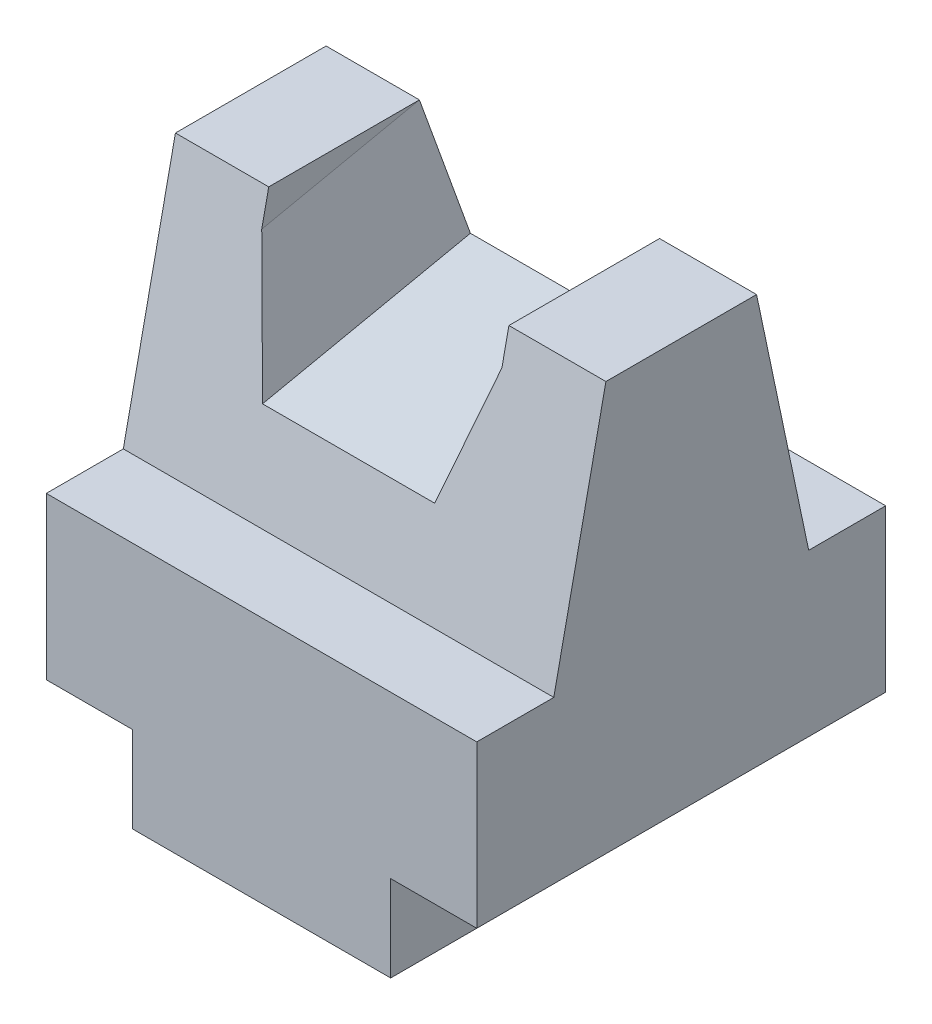
ISO-10303-21;
HEADER;
FILE_DESCRIPTION(('STEP AP214'),'2;1');
FILE_NAME('part.step','',(''),(''),'','','');
FILE_SCHEMA(('AUTOMOTIVE_DESIGN { 1 0 10303 214 1 1 1 1 }'));
ENDSEC;
DATA;
#1=APPLICATION_CONTEXT('core data for automotive mechanical design processes');
#2=APPLICATION_PROTOCOL_DEFINITION('international standard','automotive_design',2000,#1);
#3=PRODUCT_CONTEXT('',#1,'mechanical');
#4=PRODUCT('Part','Part','',(#3));
#5=PRODUCT_RELATED_PRODUCT_CATEGORY('part','',(#4));
#6=PRODUCT_DEFINITION_FORMATION('','',#4);
#7=PRODUCT_DEFINITION_CONTEXT('part definition',#1,'design');
#8=PRODUCT_DEFINITION('design','',#6,#7);
#9=PRODUCT_DEFINITION_SHAPE('','',#8);
#10=(LENGTH_UNIT() NAMED_UNIT(*) SI_UNIT(.MILLI.,.METRE.));
#11=(NAMED_UNIT(*) PLANE_ANGLE_UNIT() SI_UNIT($,.RADIAN.));
#12=(NAMED_UNIT(*) SI_UNIT($,.STERADIAN.) SOLID_ANGLE_UNIT());
#13=UNCERTAINTY_MEASURE_WITH_UNIT(LENGTH_MEASURE(1.E-05),#10,'distance_accuracy_value','');
#14=(GEOMETRIC_REPRESENTATION_CONTEXT(3) GLOBAL_UNCERTAINTY_ASSIGNED_CONTEXT((#13)) GLOBAL_UNIT_ASSIGNED_CONTEXT((#10,
#11,#12)) REPRESENTATION_CONTEXT('',''));
#15=CARTESIAN_POINT('',(0.,0.,0.));
#16=DIRECTION('',(0.,0.,1.));
#17=DIRECTION('',(1.,0.,0.));
#18=AXIS2_PLACEMENT_3D('',#15,#16,#17);
#19=CARTESIAN_POINT('',(-20.,23.,38.));
#20=DIRECTION('',(0.,-1.,0.));
#21=DIRECTION('',(0.,0.,-1.));
#22=AXIS2_PLACEMENT_3D('',#19,#20,#21);
#23=PLANE('',#22);
#24=DIRECTION('',(1.,0.,0.));
#25=VECTOR('',#24,1.);
#26=CARTESIAN_POINT('',(-20.,23.,12.));
#27=LINE('',#26,#25);
#28=CARTESIAN_POINT('',(10.9861695550396,23.,12.));
#29=VERTEX_POINT('',#28);
#30=CARTESIAN_POINT('',(20.,23.,12.));
#31=VERTEX_POINT('',#30);
#32=EDGE_CURVE('E200',#29,#31,#27,.T.);
#33=ORIENTED_EDGE('',*,*,#32,.F.);
#34=DIRECTION('',(0.,0.,1.));
#35=VECTOR('',#34,1.);
#36=CARTESIAN_POINT('',(10.9861695550396,23.,38.));
#37=LINE('',#36,#35);
#38=CARTESIAN_POINT('',(10.9861695550396,23.,26.));
#39=VERTEX_POINT('',#38);
#40=EDGE_CURVE('E167',#29,#39,#37,.T.);
#41=ORIENTED_EDGE('',*,*,#40,.T.);
#42=DIRECTION('',(-1.,0.,0.));
#43=VECTOR('',#42,1.);
#44=CARTESIAN_POINT('',(-20.,23.,26.));
#45=LINE('',#44,#43);
#46=CARTESIAN_POINT('',(20.,23.,26.));
#47=VERTEX_POINT('',#46);
#48=EDGE_CURVE('E178',#47,#39,#45,.T.);
#49=ORIENTED_EDGE('',*,*,#48,.F.);
#50=DIRECTION('',(0.,0.,-1.));
#51=VECTOR('',#50,1.);
#52=CARTESIAN_POINT('',(20.,23.,38.));
#53=LINE('',#52,#51);
#54=EDGE_CURVE('E199',#47,#31,#53,.T.);
#55=ORIENTED_EDGE('',*,*,#54,.T.);
#56=EDGE_LOOP('',(#33,#41,#49,#55));
#57=FACE_BOUND('',#56,.T.);
#58=ADVANCED_FACE('F43',(#57),#23,.F.);
#59=CARTESIAN_POINT('',(-46.,-1.44297082228117,6.85411140583554));
#60=DIRECTION('',(0.,0.206010481049842,-0.978549784986749));
#61=DIRECTION('',(0.,0.978549784986749,0.206010481049842));
#62=AXIS2_PLACEMENT_3D('',#59,#60,#61);
#63=PLANE('',#62);
#64=DIRECTION('',(-1.,0.,0.));
#65=VECTOR('',#64,1.);
#66=CARTESIAN_POINT('',(-46.,12.4045745886902,9.76938412393479));
#67=LINE('',#66,#65);
#68=CARTESIAN_POINT('',(7.18004102876759,12.4045745886902,9.76938412393478));
#69=VERTEX_POINT('',#68);
#70=CARTESIAN_POINT('',(-8.81995897123242,12.4045745886902,9.76938412393479));
#71=VERTEX_POINT('',#70);
#72=EDGE_CURVE('E279',#69,#71,#67,.T.);
#73=ORIENTED_EDGE('',*,*,#72,.F.);
#74=DIRECTION('',(0.331626211396949,0.923174496877331,0.194352525658385));
#75=VECTOR('',#74,1.);
#76=CARTESIAN_POINT('',(-3.09579074243356,-16.2010829237665,3.74714043710179));
#77=LINE('',#76,#75);
#78=EDGE_CURVE('E286',#69,#29,#77,.T.);
#79=ORIENTED_EDGE('',*,*,#78,.T.);
#80=ORIENTED_EDGE('',*,*,#32,.T.);
#81=DIRECTION('',(0.,-0.978549784986749,-0.206010481049842));
#82=VECTOR('',#81,1.);
#83=CARTESIAN_POINT('',(20.,28.2413793103448,13.1034482758621));
#84=LINE('',#83,#82);
#85=CARTESIAN_POINT('',(20.,0.,7.15789473684211));
#86=VERTEX_POINT('',#85);
#87=EDGE_CURVE('E271',#31,#86,#84,.T.);
#88=ORIENTED_EDGE('',*,*,#87,.T.);
#89=DIRECTION('',(1.,0.,0.));
#90=VECTOR('',#89,1.);
#91=CARTESIAN_POINT('',(-46.,0.,7.15789473684211));
#92=LINE('',#91,#90);
#93=CARTESIAN_POINT('',(-20.,0.,7.15789473684211));
#94=VERTEX_POINT('',#93);
#95=EDGE_CURVE('E273',#94,#86,#92,.T.);
#96=ORIENTED_EDGE('',*,*,#95,.F.);
#97=DIRECTION('',(0.,0.978549784986749,0.206010481049842));
#98=VECTOR('',#97,1.);
#99=CARTESIAN_POINT('',(-20.,28.2413793103448,13.1034482758621));
#100=LINE('',#99,#98);
#101=CARTESIAN_POINT('',(-20.,23.,12.));
#102=VERTEX_POINT('',#101);
#103=EDGE_CURVE('E267',#94,#102,#100,.T.);
#104=ORIENTED_EDGE('',*,*,#103,.T.);
#105=CARTESIAN_POINT('',(-11.3311099886057,23.,12.0000000000001));
#106=VERTEX_POINT('',#105);
#107=EDGE_CURVE('E198',#102,#106,#27,.T.);
#108=ORIENTED_EDGE('',*,*,#107,.T.);
#109=DIRECTION('',(-0.225923291600866,0.953249473358433,0.200684099654407));
#110=VECTOR('',#109,1.);
#111=CARTESIAN_POINT('',(-7.60327687289893,7.27096679968001,8.68862458940632));
#112=LINE('',#111,#110);
#113=EDGE_CURVE('E289',#71,#106,#112,.T.);
#114=ORIENTED_EDGE('',*,*,#113,.F.);
#115=EDGE_LOOP('',(#73,#79,#80,#88,#96,#104,#108,#114));
#116=FACE_BOUND('',#115,.T.);
#117=ADVANCED_FACE('F308',(#116),#63,.T.);
#118=CARTESIAN_POINT('',(-20.,23.,38.));
#119=DIRECTION('',(1.,0.,0.));
#120=DIRECTION('',(0.,1.,0.));
#121=AXIS2_PLACEMENT_3D('',#118,#119,#120);
#122=PLANE('',#121);
#123=DIRECTION('',(0.,-0.978549784986749,0.206010481049842));
#124=VECTOR('',#123,1.);
#125=CARTESIAN_POINT('',(-20.,20.5809018567639,26.5092838196287));
#126=LINE('',#125,#124);
#127=CARTESIAN_POINT('',(-20.,23.,26.));
#128=VERTEX_POINT('',#127);
#129=CARTESIAN_POINT('',(-20.,0.,30.8421052631579));
#130=VERTEX_POINT('',#129);
#131=EDGE_CURVE('E264',#128,#130,#126,.T.);
#132=ORIENTED_EDGE('',*,*,#131,.F.);
#133=DIRECTION('',(0.,0.,-1.));
#134=VECTOR('',#133,1.);
#135=CARTESIAN_POINT('',(-20.,23.,38.));
#136=LINE('',#135,#134);
#137=EDGE_CURVE('E201',#128,#102,#136,.T.);
#138=ORIENTED_EDGE('',*,*,#137,.T.);
#139=ORIENTED_EDGE('',*,*,#103,.F.);
#140=DIRECTION('',(0.,0.,-1.));
#141=VECTOR('',#140,1.);
#142=CARTESIAN_POINT('',(-20.,0.,38.));
#143=LINE('',#142,#141);
#144=CARTESIAN_POINT('',(-20.,0.,0.));
#145=VERTEX_POINT('',#144);
#146=EDGE_CURVE('E265',#94,#145,#143,.T.);
#147=ORIENTED_EDGE('',*,*,#146,.T.);
#148=DIRECTION('',(0.,-1.,0.));
#149=VECTOR('',#148,1.);
#150=CARTESIAN_POINT('',(-20.,23.,0.));
#151=LINE('',#150,#149);
#152=CARTESIAN_POINT('',(-20.,-15.,0.));
#153=VERTEX_POINT('',#152);
#154=EDGE_CURVE('E211',#145,#153,#151,.T.);
#155=ORIENTED_EDGE('',*,*,#154,.T.);
#156=DIRECTION('',(0.,0.,1.));
#157=VECTOR('',#156,1.);
#158=CARTESIAN_POINT('',(-20.,-15.,0.));
#159=LINE('',#158,#157);
#160=CARTESIAN_POINT('',(-20.,-15.,38.));
#161=VERTEX_POINT('',#160);
#162=EDGE_CURVE('E224',#153,#161,#159,.T.);
#163=ORIENTED_EDGE('',*,*,#162,.T.);
#164=DIRECTION('',(0.,-1.,0.));
#165=VECTOR('',#164,1.);
#166=CARTESIAN_POINT('',(-20.,23.,38.));
#167=LINE('',#166,#165);
#168=CARTESIAN_POINT('',(-20.,0.,38.));
#169=VERTEX_POINT('',#168);
#170=EDGE_CURVE('E218',#169,#161,#167,.T.);
#171=ORIENTED_EDGE('',*,*,#170,.F.);
#172=DIRECTION('',(0.,0.,-1.));
#173=VECTOR('',#172,1.);
#174=CARTESIAN_POINT('',(-20.,0.,38.));
#175=LINE('',#174,#173);
#176=EDGE_CURVE('E254',#169,#130,#175,.T.);
#177=ORIENTED_EDGE('',*,*,#176,.T.);
#178=EDGE_LOOP('',(#132,#138,#139,#147,#155,#163,#171,#177));
#179=FACE_BOUND('',#178,.T.);
#180=ADVANCED_FACE('F313',(#179),#122,.F.);
#181=CARTESIAN_POINT('',(20.,23.,38.));
#182=DIRECTION('',(-1.,0.,0.));
#183=DIRECTION('',(0.,-1.,0.));
#184=AXIS2_PLACEMENT_3D('',#181,#182,#183);
#185=PLANE('',#184);
#186=DIRECTION('',(0.,0.978549784986749,-0.206010481049842));
#187=VECTOR('',#186,1.);
#188=CARTESIAN_POINT('',(20.,20.5809018567639,26.5092838196287));
#189=LINE('',#188,#187);
#190=CARTESIAN_POINT('',(20.,0.,30.8421052631579));
#191=VERTEX_POINT('',#190);
#192=EDGE_CURVE('E270',#191,#47,#189,.T.);
#193=ORIENTED_EDGE('',*,*,#192,.F.);
#194=DIRECTION('',(0.,0.,1.));
#195=VECTOR('',#194,1.);
#196=CARTESIAN_POINT('',(20.,0.,38.));
#197=LINE('',#196,#195);
#198=CARTESIAN_POINT('',(20.,0.,38.));
#199=VERTEX_POINT('',#198);
#200=EDGE_CURVE('E188',#191,#199,#197,.T.);
#201=ORIENTED_EDGE('',*,*,#200,.T.);
#202=DIRECTION('',(0.,1.,0.));
#203=VECTOR('',#202,1.);
#204=CARTESIAN_POINT('',(20.,23.,38.));
#205=LINE('',#204,#203);
#206=CARTESIAN_POINT('',(20.,-15.,38.));
#207=VERTEX_POINT('',#206);
#208=EDGE_CURVE('E209',#207,#199,#205,.T.);
#209=ORIENTED_EDGE('',*,*,#208,.F.);
#210=DIRECTION('',(0.,0.,1.));
#211=VECTOR('',#210,1.);
#212=CARTESIAN_POINT('',(20.,-15.,0.));
#213=LINE('',#212,#211);
#214=CARTESIAN_POINT('',(20.,-15.,0.));
#215=VERTEX_POINT('',#214);
#216=EDGE_CURVE('E245',#215,#207,#213,.T.);
#217=ORIENTED_EDGE('',*,*,#216,.F.);
#218=DIRECTION('',(0.,1.,0.));
#219=VECTOR('',#218,1.);
#220=CARTESIAN_POINT('',(20.,23.,0.));
#221=LINE('',#220,#219);
#222=CARTESIAN_POINT('',(20.,0.,0.));
#223=VERTEX_POINT('',#222);
#224=EDGE_CURVE('E213',#215,#223,#221,.T.);
#225=ORIENTED_EDGE('',*,*,#224,.T.);
#226=DIRECTION('',(0.,0.,1.));
#227=VECTOR('',#226,1.);
#228=CARTESIAN_POINT('',(20.,0.,38.));
#229=LINE('',#228,#227);
#230=EDGE_CURVE('E191',#223,#86,#229,.T.);
#231=ORIENTED_EDGE('',*,*,#230,.T.);
#232=ORIENTED_EDGE('',*,*,#87,.F.);
#233=ORIENTED_EDGE('',*,*,#54,.F.);
#234=EDGE_LOOP('',(#193,#201,#209,#217,#225,#231,#232,#233));
#235=FACE_BOUND('',#234,.T.);
#236=ADVANCED_FACE('F44',(#235),#185,.F.);
#237=CARTESIAN_POINT('',(-11.3311099886057,23.,26.));
#238=VERTEX_POINT('',#237);
#239=EDGE_CURVE('E195',#238,#128,#45,.T.);
#240=ORIENTED_EDGE('',*,*,#239,.F.);
#241=DIRECTION('',(0.,0.,-1.));
#242=VECTOR('',#241,1.);
#243=CARTESIAN_POINT('',(-11.3311099886057,23.,38.));
#244=LINE('',#243,#242);
#245=EDGE_CURVE('E180',#238,#106,#244,.T.);
#246=ORIENTED_EDGE('',*,*,#245,.T.);
#247=ORIENTED_EDGE('',*,*,#107,.F.);
#248=ORIENTED_EDGE('',*,*,#137,.F.);
#249=EDGE_LOOP('',(#240,#246,#247,#248));
#250=FACE_BOUND('',#249,.T.);
#251=ADVANCED_FACE('F297',(#250),#23,.F.);
#252=CARTESIAN_POINT('',(0.,0.,38.));
#253=DIRECTION('',(0.,0.,1.));
#254=DIRECTION('',(1.,0.,0.));
#255=AXIS2_PLACEMENT_3D('',#252,#253,#254);
#256=PLANE('',#255);
#257=DIRECTION('',(1.,0.,0.));
#258=VECTOR('',#257,1.);
#259=CARTESIAN_POINT('',(-46.,0.,38.));
#260=LINE('',#259,#258);
#261=EDGE_CURVE('E283',#169,#199,#260,.T.);
#262=ORIENTED_EDGE('',*,*,#261,.F.);
#263=ORIENTED_EDGE('',*,*,#170,.T.);
#264=DIRECTION('',(1.,0.,0.));
#265=VECTOR('',#264,1.);
#266=CARTESIAN_POINT('',(0.,-15.,38.));
#267=LINE('',#266,#265);
#268=CARTESIAN_POINT('',(-12.,-15.,38.));
#269=VERTEX_POINT('',#268);
#270=EDGE_CURVE('E233',#161,#269,#267,.T.);
#271=ORIENTED_EDGE('',*,*,#270,.T.);
#272=DIRECTION('',(0.,1.,0.));
#273=VECTOR('',#272,1.);
#274=CARTESIAN_POINT('',(-12.,0.,38.));
#275=LINE('',#274,#273);
#276=CARTESIAN_POINT('',(-12.,-23.,38.));
#277=VERTEX_POINT('',#276);
#278=EDGE_CURVE('E229',#277,#269,#275,.T.);
#279=ORIENTED_EDGE('',*,*,#278,.F.);
#280=DIRECTION('',(1.,0.,0.));
#281=VECTOR('',#280,1.);
#282=CARTESIAN_POINT('',(-20.,-23.,38.));
#283=LINE('',#282,#281);
#284=CARTESIAN_POINT('',(12.,-23.,38.));
#285=VERTEX_POINT('',#284);
#286=EDGE_CURVE('E206',#277,#285,#283,.T.);
#287=ORIENTED_EDGE('',*,*,#286,.T.);
#288=DIRECTION('',(0.,-1.,0.));
#289=VECTOR('',#288,1.);
#290=CARTESIAN_POINT('',(12.,-23.,38.));
#291=LINE('',#290,#289);
#292=CARTESIAN_POINT('',(12.,-15.,38.));
#293=VERTEX_POINT('',#292);
#294=EDGE_CURVE('E248',#293,#285,#291,.T.);
#295=ORIENTED_EDGE('',*,*,#294,.F.);
#296=DIRECTION('',(-1.,0.,0.));
#297=VECTOR('',#296,1.);
#298=CARTESIAN_POINT('',(12.,-15.,38.));
#299=LINE('',#298,#297);
#300=EDGE_CURVE('E252',#207,#293,#299,.T.);
#301=ORIENTED_EDGE('',*,*,#300,.F.);
#302=ORIENTED_EDGE('',*,*,#208,.T.);
#303=EDGE_LOOP('',(#262,#263,#271,#279,#287,#295,#301,#302));
#304=FACE_BOUND('',#303,.T.);
#305=ADVANCED_FACE('F324',(#304),#256,.T.);
#306=CARTESIAN_POINT('',(0.,0.,0.));
#307=DIRECTION('',(0.,0.,1.));
#308=DIRECTION('',(1.,0.,0.));
#309=AXIS2_PLACEMENT_3D('',#306,#307,#308);
#310=PLANE('',#309);
#311=ORIENTED_EDGE('',*,*,#154,.F.);
#312=DIRECTION('',(1.,0.,0.));
#313=VECTOR('',#312,1.);
#314=CARTESIAN_POINT('',(-46.,0.,0.));
#315=LINE('',#314,#313);
#316=EDGE_CURVE('E280',#145,#223,#315,.T.);
#317=ORIENTED_EDGE('',*,*,#316,.T.);
#318=ORIENTED_EDGE('',*,*,#224,.F.);
#319=DIRECTION('',(-1.,0.,0.));
#320=VECTOR('',#319,1.);
#321=CARTESIAN_POINT('',(12.,-15.,0.));
#322=LINE('',#321,#320);
#323=CARTESIAN_POINT('',(12.,-15.,0.));
#324=VERTEX_POINT('',#323);
#325=EDGE_CURVE('E253',#215,#324,#322,.T.);
#326=ORIENTED_EDGE('',*,*,#325,.T.);
#327=DIRECTION('',(0.,-1.,0.));
#328=VECTOR('',#327,1.);
#329=CARTESIAN_POINT('',(12.,-23.,0.));
#330=LINE('',#329,#328);
#331=CARTESIAN_POINT('',(12.,-23.,0.));
#332=VERTEX_POINT('',#331);
#333=EDGE_CURVE('E244',#324,#332,#330,.T.);
#334=ORIENTED_EDGE('',*,*,#333,.T.);
#335=DIRECTION('',(1.,0.,0.));
#336=VECTOR('',#335,1.);
#337=CARTESIAN_POINT('',(-20.,-23.,0.));
#338=LINE('',#337,#336);
#339=CARTESIAN_POINT('',(-12.,-23.,0.));
#340=VERTEX_POINT('',#339);
#341=EDGE_CURVE('E210',#340,#332,#338,.T.);
#342=ORIENTED_EDGE('',*,*,#341,.F.);
#343=DIRECTION('',(0.,1.,0.));
#344=VECTOR('',#343,1.);
#345=CARTESIAN_POINT('',(-12.,0.,0.));
#346=LINE('',#345,#344);
#347=CARTESIAN_POINT('',(-12.,-15.,0.));
#348=VERTEX_POINT('',#347);
#349=EDGE_CURVE('E230',#340,#348,#346,.T.);
#350=ORIENTED_EDGE('',*,*,#349,.T.);
#351=DIRECTION('',(1.,0.,0.));
#352=VECTOR('',#351,1.);
#353=CARTESIAN_POINT('',(0.,-15.,0.));
#354=LINE('',#353,#352);
#355=EDGE_CURVE('E234',#153,#348,#354,.T.);
#356=ORIENTED_EDGE('',*,*,#355,.F.);
#357=EDGE_LOOP('',(#311,#317,#318,#326,#334,#342,#350,#356));
#358=FACE_BOUND('',#357,.T.);
#359=ADVANCED_FACE('F335',(#358),#310,.F.);
#360=CARTESIAN_POINT('',(-20.,-23.,38.));
#361=DIRECTION('',(0.,1.,0.));
#362=DIRECTION('',(0.,0.,1.));
#363=AXIS2_PLACEMENT_3D('',#360,#361,#362);
#364=PLANE('',#363);
#365=ORIENTED_EDGE('',*,*,#341,.T.);
#366=DIRECTION('',(0.,0.,1.));
#367=VECTOR('',#366,1.);
#368=CARTESIAN_POINT('',(12.,-23.,0.));
#369=LINE('',#368,#367);
#370=EDGE_CURVE('E240',#332,#285,#369,.T.);
#371=ORIENTED_EDGE('',*,*,#370,.T.);
#372=ORIENTED_EDGE('',*,*,#286,.F.);
#373=DIRECTION('',(0.,0.,1.));
#374=VECTOR('',#373,1.);
#375=CARTESIAN_POINT('',(-12.,-23.,0.));
#376=LINE('',#375,#374);
#377=EDGE_CURVE('E228',#340,#277,#376,.T.);
#378=ORIENTED_EDGE('',*,*,#377,.F.);
#379=EDGE_LOOP('',(#365,#371,#372,#378));
#380=FACE_BOUND('',#379,.T.);
#381=ADVANCED_FACE('F367',(#380),#364,.F.);
#382=CARTESIAN_POINT('',(0.,-15.,0.));
#383=DIRECTION('',(0.,-1.,0.));
#384=DIRECTION('',(0.,0.,-1.));
#385=AXIS2_PLACEMENT_3D('',#382,#383,#384);
#386=PLANE('',#385);
#387=ORIENTED_EDGE('',*,*,#270,.F.);
#388=ORIENTED_EDGE('',*,*,#162,.F.);
#389=ORIENTED_EDGE('',*,*,#355,.T.);
#390=DIRECTION('',(0.,0.,1.));
#391=VECTOR('',#390,1.);
#392=CARTESIAN_POINT('',(-12.,-15.,0.));
#393=LINE('',#392,#391);
#394=EDGE_CURVE('E216',#348,#269,#393,.T.);
#395=ORIENTED_EDGE('',*,*,#394,.T.);
#396=EDGE_LOOP('',(#387,#388,#389,#395));
#397=FACE_BOUND('',#396,.T.);
#398=ADVANCED_FACE('F373',(#397),#386,.T.);
#399=CARTESIAN_POINT('',(-12.,0.,0.));
#400=DIRECTION('',(1.,0.,0.));
#401=DIRECTION('',(0.,0.,-1.));
#402=AXIS2_PLACEMENT_3D('',#399,#400,#401);
#403=PLANE('',#402);
#404=ORIENTED_EDGE('',*,*,#278,.T.);
#405=ORIENTED_EDGE('',*,*,#394,.F.);
#406=ORIENTED_EDGE('',*,*,#349,.F.);
#407=ORIENTED_EDGE('',*,*,#377,.T.);
#408=EDGE_LOOP('',(#404,#405,#406,#407));
#409=FACE_BOUND('',#408,.T.);
#410=ADVANCED_FACE('F377',(#409),#403,.F.);
#411=CARTESIAN_POINT('',(12.,-23.,0.));
#412=DIRECTION('',(-1.,0.,0.));
#413=DIRECTION('',(0.,0.,1.));
#414=AXIS2_PLACEMENT_3D('',#411,#412,#413);
#415=PLANE('',#414);
#416=ORIENTED_EDGE('',*,*,#294,.T.);
#417=ORIENTED_EDGE('',*,*,#370,.F.);
#418=ORIENTED_EDGE('',*,*,#333,.F.);
#419=DIRECTION('',(0.,0.,1.));
#420=VECTOR('',#419,1.);
#421=CARTESIAN_POINT('',(12.,-15.,0.));
#422=LINE('',#421,#420);
#423=EDGE_CURVE('E242',#324,#293,#422,.T.);
#424=ORIENTED_EDGE('',*,*,#423,.T.);
#425=EDGE_LOOP('',(#416,#417,#418,#424));
#426=FACE_BOUND('',#425,.T.);
#427=ADVANCED_FACE('F382',(#426),#415,.F.);
#428=CARTESIAN_POINT('',(12.,-15.,0.));
#429=DIRECTION('',(0.,1.,0.));
#430=DIRECTION('',(0.,0.,1.));
#431=AXIS2_PLACEMENT_3D('',#428,#429,#430);
#432=PLANE('',#431);
#433=ORIENTED_EDGE('',*,*,#300,.T.);
#434=ORIENTED_EDGE('',*,*,#423,.F.);
#435=ORIENTED_EDGE('',*,*,#325,.F.);
#436=ORIENTED_EDGE('',*,*,#216,.T.);
#437=EDGE_LOOP('',(#433,#434,#435,#436));
#438=FACE_BOUND('',#437,.T.);
#439=ADVANCED_FACE('F327',(#438),#432,.F.);
#440=CARTESIAN_POINT('',(-46.,0.,0.));
#441=DIRECTION('',(0.,-1.,0.));
#442=DIRECTION('',(0.,0.,-1.));
#443=AXIS2_PLACEMENT_3D('',#440,#441,#442);
#444=PLANE('',#443);
#445=ORIENTED_EDGE('',*,*,#95,.T.);
#446=ORIENTED_EDGE('',*,*,#230,.F.);
#447=ORIENTED_EDGE('',*,*,#316,.F.);
#448=ORIENTED_EDGE('',*,*,#146,.F.);
#449=EDGE_LOOP('',(#445,#446,#447,#448));
#450=FACE_BOUND('',#449,.T.);
#451=ADVANCED_FACE('F333',(#450),#444,.F.);
#452=CARTESIAN_POINT('',(-46.,0.,0.));
#453=DIRECTION('',(0.,-1.,0.));
#454=DIRECTION('',(0.,0.,-1.));
#455=AXIS2_PLACEMENT_3D('',#452,#453,#454);
#456=PLANE('',#455);
#457=ORIENTED_EDGE('',*,*,#261,.T.);
#458=ORIENTED_EDGE('',*,*,#200,.F.);
#459=DIRECTION('',(1.,0.,0.));
#460=VECTOR('',#459,1.);
#461=CARTESIAN_POINT('',(-46.,0.,30.8421052631579));
#462=LINE('',#461,#460);
#463=EDGE_CURVE('E272',#130,#191,#462,.T.);
#464=ORIENTED_EDGE('',*,*,#463,.F.);
#465=ORIENTED_EDGE('',*,*,#176,.F.);
#466=EDGE_LOOP('',(#457,#458,#464,#465));
#467=FACE_BOUND('',#466,.T.);
#468=ADVANCED_FACE('F320',(#467),#456,.F.);
#469=CARTESIAN_POINT('',(-46.,6.21750663129974,29.5331564986737));
#470=DIRECTION('',(0.,0.206010481049842,0.978549784986749));
#471=DIRECTION('',(0.,-0.978549784986749,0.206010481049842));
#472=AXIS2_PLACEMENT_3D('',#469,#470,#471);
#473=PLANE('',#472);
#474=DIRECTION('',(0.,0.978549784986749,-0.206010481049842));
#475=VECTOR('',#474,1.);
#476=CARTESIAN_POINT('',(10.9861695550396,6.21750663129974,29.5331564986737));
#477=LINE('',#476,#475);
#478=CARTESIAN_POINT('',(10.9861695550396,19.9159420289855,26.6492753623189));
#479=VERTEX_POINT('',#478);
#480=EDGE_CURVE('E163',#479,#39,#477,.T.);
#481=ORIENTED_EDGE('',*,*,#480,.F.);
#482=DIRECTION('',(-0.306227170808341,-0.931538751639651,0.196113421397821));
#483=VECTOR('',#482,1.);
#484=CARTESIAN_POINT('',(1.56144510730515,-8.75393734003065,32.6850394400065));
#485=LINE('',#484,#483);
#486=CARTESIAN_POINT('',(7.18004102876758,8.33775252155425,29.0867889428307));
#487=VERTEX_POINT('',#486);
#488=EDGE_CURVE('E51',#479,#487,#485,.T.);
#489=ORIENTED_EDGE('',*,*,#488,.T.);
#490=DIRECTION('',(1.,0.,0.));
#491=VECTOR('',#490,1.);
#492=CARTESIAN_POINT('',(-46.,8.33775252155425,29.0867889428307));
#493=LINE('',#492,#491);
#494=CARTESIAN_POINT('',(-8.81995897123242,8.33775252155425,29.0867889428307));
#495=VERTEX_POINT('',#494);
#496=EDGE_CURVE('E11',#495,#487,#493,.T.);
#497=ORIENTED_EDGE('',*,*,#496,.F.);
#498=DIRECTION('',(0.207609852951133,-0.957228858180155,0.201521864880033));
#499=VECTOR('',#498,1.);
#500=CARTESIAN_POINT('',(-9.98245570132067,13.6976880051677,27.9583814725963));
#501=LINE('',#500,#499);
#502=CARTESIAN_POINT('',(-11.3311099886057,19.9159420289855,26.6492753623188));
#503=VERTEX_POINT('',#502);
#504=EDGE_CURVE('E183',#503,#495,#501,.T.);
#505=ORIENTED_EDGE('',*,*,#504,.F.);
#506=DIRECTION('',(0.,-0.978549784986749,0.206010481049842));
#507=VECTOR('',#506,1.);
#508=CARTESIAN_POINT('',(-11.3311099886057,6.21750663129974,29.5331564986737));
#509=LINE('',#508,#507);
#510=EDGE_CURVE('E66',#238,#503,#509,.T.);
#511=ORIENTED_EDGE('',*,*,#510,.F.);
#512=ORIENTED_EDGE('',*,*,#239,.T.);
#513=ORIENTED_EDGE('',*,*,#131,.T.);
#514=ORIENTED_EDGE('',*,*,#463,.T.);
#515=ORIENTED_EDGE('',*,*,#192,.T.);
#516=ORIENTED_EDGE('',*,*,#48,.T.);
#517=EDGE_LOOP('',(#481,#489,#497,#505,#511,#512,#513,#514,#515,#516));
#518=FACE_BOUND('',#517,.T.);
#519=ADVANCED_FACE('F176',(#518),#473,.T.);
#520=CARTESIAN_POINT('',(0.,2.9280924603975,54.7826742333253));
#521=DIRECTION('',(0.,-0.978549784986749,-0.206010481049842));
#522=DIRECTION('',(0.,0.206010481049842,-0.978549784986749));
#523=AXIS2_PLACEMENT_3D('',#520,#521,#522);
#524=PLANE('',#523);
#525=ORIENTED_EDGE('',*,*,#72,.T.);
#526=DIRECTION('',(0.,0.206010481049842,-0.978549784986749));
#527=VECTOR('',#526,1.);
#528=CARTESIAN_POINT('',(-8.81995897123242,2.9280924603975,54.7826742333253));
#529=LINE('',#528,#527);
#530=EDGE_CURVE('E59',#495,#71,#529,.T.);
#531=ORIENTED_EDGE('',*,*,#530,.F.);
#532=ORIENTED_EDGE('',*,*,#496,.T.);
#533=DIRECTION('',(0.,0.206010481049842,-0.978549784986749));
#534=VECTOR('',#533,1.);
#535=CARTESIAN_POINT('',(7.18004102876758,2.9280924603975,54.7826742333253));
#536=LINE('',#535,#534);
#537=EDGE_CURVE('E168',#487,#69,#536,.T.);
#538=ORIENTED_EDGE('',*,*,#537,.T.);
#539=EDGE_LOOP('',(#525,#531,#532,#538));
#540=FACE_BOUND('',#539,.T.);
#541=ADVANCED_FACE('F339',(#540),#524,.F.);
#542=CARTESIAN_POINT('',(1.96310268549916,-11.5947174526044,51.7252405674301));
#543=DIRECTION('',(-0.943410862728698,0.324512757858455,0.0683184753386221));
#544=DIRECTION('',(-0.325272736954854,-0.945620244386666,0.));
#545=AXIS2_PLACEMENT_3D('',#542,#543,#544);
#546=PLANE('',#545);
#547=ORIENTED_EDGE('',*,*,#537,.F.);
#548=ORIENTED_EDGE('',*,*,#488,.F.);
#549=DIRECTION('',(0.,0.206010481049842,-0.978549784986749));
#550=VECTOR('',#549,1.);
#551=CARTESIAN_POINT('',(10.9861695550396,13.5235178717073,57.0132901093905));
#552=LINE('',#551,#550);
#553=EDGE_CURVE('E161',#479,#29,#552,.T.);
#554=ORIENTED_EDGE('',*,*,#553,.T.);
#555=ORIENTED_EDGE('',*,*,#78,.F.);
#556=EDGE_LOOP('',(#547,#548,#554,#555));
#557=FACE_BOUND('',#556,.T.);
#558=ADVANCED_FACE('F181',(#557),#546,.T.);
#559=CARTESIAN_POINT('',(-5.25537552326151,-12.1121332305575,51.6163109299663));
#560=DIRECTION('',(-0.974145095102485,-0.221077188419526,-0.0465425659830581));
#561=DIRECTION('',(0.22131702800492,-0.975201914023485,0.));
#562=AXIS2_PLACEMENT_3D('',#559,#560,#561);
#563=PLANE('',#562);
#564=ORIENTED_EDGE('',*,*,#113,.T.);
#565=DIRECTION('',(0.,0.206010481049842,-0.978549784986749));
#566=VECTOR('',#565,1.);
#567=CARTESIAN_POINT('',(-11.3311099886057,13.5235178717073,57.0132901093905));
#568=LINE('',#567,#566);
#569=EDGE_CURVE('E173',#503,#106,#568,.T.);
#570=ORIENTED_EDGE('',*,*,#569,.F.);
#571=ORIENTED_EDGE('',*,*,#504,.T.);
#572=ORIENTED_EDGE('',*,*,#530,.T.);
#573=EDGE_LOOP('',(#564,#570,#571,#572));
#574=FACE_BOUND('',#573,.T.);
#575=ADVANCED_FACE('F302',(#574),#563,.F.);
#576=CARTESIAN_POINT('',(-11.3311099886057,13.5235178717073,57.0132901093905));
#577=DIRECTION('',(-1.,0.,0.));
#578=DIRECTION('',(0.,0.,1.));
#579=AXIS2_PLACEMENT_3D('',#576,#577,#578);
#580=PLANE('',#579);
#581=ORIENTED_EDGE('',*,*,#510,.T.);
#582=ORIENTED_EDGE('',*,*,#569,.T.);
#583=ORIENTED_EDGE('',*,*,#245,.F.);
#584=EDGE_LOOP('',(#581,#582,#583));
#585=FACE_BOUND('',#584,.T.);
#586=ADVANCED_FACE('F492',(#585),#580,.F.);
#587=CARTESIAN_POINT('',(10.9861695550396,13.5235178717073,57.0132901093905));
#588=DIRECTION('',(1.,0.,0.));
#589=DIRECTION('',(0.,0.,-1.));
#590=AXIS2_PLACEMENT_3D('',#587,#588,#589);
#591=PLANE('',#590);
#592=ORIENTED_EDGE('',*,*,#553,.F.);
#593=ORIENTED_EDGE('',*,*,#480,.T.);
#594=ORIENTED_EDGE('',*,*,#40,.F.);
#595=EDGE_LOOP('',(#592,#593,#594));
#596=FACE_BOUND('',#595,.T.);
#597=ADVANCED_FACE('F162',(#596),#591,.F.);
#598=CLOSED_SHELL('',(#58,#117,#180,#236,#251,#305,#359,#381,#398,#410,#427,#439,#451,#468,#519,
#541,#558,#575,#586,#597));
#599=MANIFOLD_SOLID_BREP('B2',#598);
#600=ADVANCED_BREP_SHAPE_REPRESENTATION('',(#18,#599),#14);
#601=SHAPE_DEFINITION_REPRESENTATION(#9,#600);
ENDSEC;
END-ISO-10303-21;
